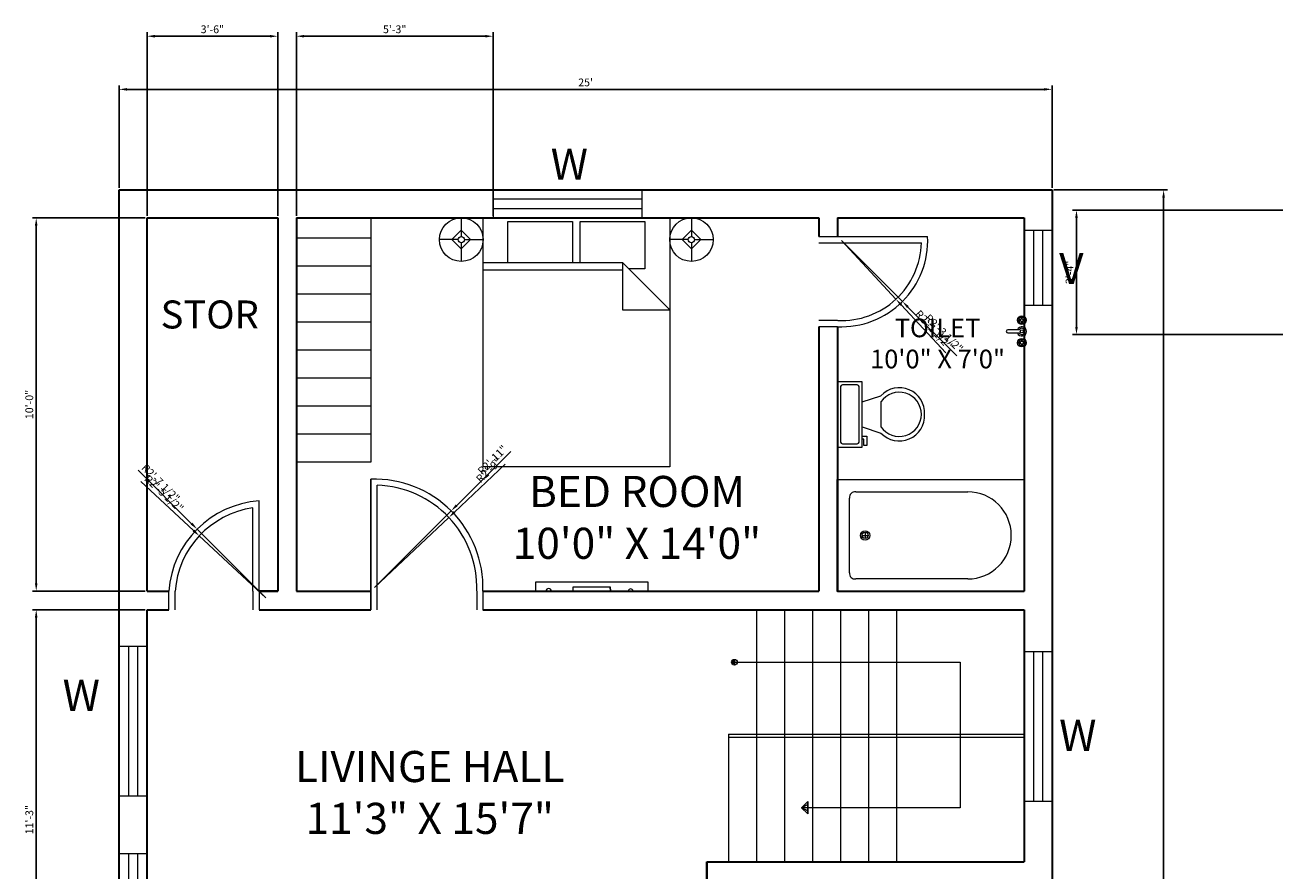
# Model space of a CAD drawing. Units: inches. Extents: x 2318 to 3542, y 1525 to 2117.
# Tile 4 of 6: x 2767 to 3169, y 1816 to 2088. Entities that reach past the tile are written whole.
import ezdxf

# ---------------------------------------------------------------- set-up
doc = ezdxf.new("R2010")
doc.units = ezdxf.units.IN
for name, color, linetype, lineweight in [('A-ANNO-DIMS', 2, 'Continuous', 18), ('A-ANNO-SYMB', 2, 'Continuous', 13), ('A-ANNO-TEXT', 7, 'Continuous', 18), ('A-AREA-IDEN', 7, 'Continuous', 25), ('A-DOOR', 4, 'Continuous', 18), ('A-EQPM', 9, 'Continuous', 18), ('A-FLOR-CASE', 8, 'Continuous', 18), ('A-FLOR-FIXT', 9, 'Continuous', 18), ('A-FLOR-STRS', 3, 'Continuous', 18), ('A-FURN', 8, 'Continuous', 18), ('A-GLAZ', 4, 'Continuous', 18), ('A-WALL', 7, 'Continuous', 35)]:
    doc.layers.add(name, color=color, linetype=linetype, lineweight=lineweight)
doc.styles.add('Annotative', font='arial.ttf')
doc.styles.get("Standard").update_dxf_attribs({"font": 'arial.ttf'})
doc.dimstyles.new('ISO-25', dxfattribs={"dimtxt": 2.5, "dimasz": 2.5, "dimexe": 1.25, "dimexo": 0.625, "dimtad": 1, "dimdec": 0, "dimlunit": 3, "dimtxsty": 'Standard', "dimcen": 2.5, "dimadec": 0, "dimazin": 0, "dimtfac": 1, "dimtdec": 0, "dimtmove": 0, "dimatfit": 3, "dimfxl": 1, "dimarcsym": 0})

# ---------------------------------------------------------------- blocks, each defined once
blk = doc.blocks.new('*D17')
at = {"layer": 'A-ANNO-DIMS', "color": 0, "lineweight": -2, "transparency": 16777216}
for p, q in [((2797.41, 2035.22), (2797.41, 2068.17)), ((2799.91, 2066.92), (3094.91, 2066.92)), ((3097.41, 2035.22), (3097.41, 2068.17))]:
    blk.add_line(p, q, dxfattribs=at)
at = {"layer": 'A-ANNO-DIMS', "color": 0, "transparency": 16777216}
for points in [[(2799.91, 2067.33), (2799.91, 2066.5), (2797.41, 2066.92)], [(3094.91, 2067.33), (3094.91, 2066.5), (3097.41, 2066.92)]]:
    blk.add_solid(points, dxfattribs=at)
at = {"layer": 'Defpoints', "color": 0, "transparency": 16777216}
for p in [(3097.41, 2066.92), (2797.41, 2034.59), (3097.41, 2034.59)]:
    blk.add_point(p, dxfattribs=at)
at = {"layer": 'A-ANNO-DIMS', "color": 0, "transparency": 16777216, "insert": (2947.41, 2068.82), "char_height": 2.5, "attachment_point": 5}
blk.add_mtext("25'", dxfattribs=at)
blk = doc.blocks.new('*D18')
at = {"layer": 'A-ANNO-DIMS', "color": 0, "lineweight": -2, "transparency": 16777216}
for p, q in [((3098.03, 2034.59), (3134.53, 2034.59)), ((3133.28, 2032.09), (3133.28, 1557.09)), ((3098.03, 1554.59), (3134.53, 1554.59))]:
    blk.add_line(p, q, dxfattribs=at)
at = {"layer": 'A-ANNO-DIMS', "color": 0, "transparency": 16777216}
for points in [[(3132.86, 2032.09), (3133.69, 2032.09), (3133.28, 2034.59)], [(3132.86, 1557.09), (3133.69, 1557.09), (3133.28, 1554.59)]]:
    blk.add_solid(points, dxfattribs=at)
at = {"layer": 'Defpoints', "color": 0, "transparency": 16777216}
for p in [(3097.41, 2034.59), (3097.41, 1554.59), (3133.28, 1554.59)]:
    blk.add_point(p, dxfattribs=at)
at = {"layer": 'A-ANNO-DIMS', "color": 0, "transparency": 16777216, "insert": (3131.38, 1794.59), "char_height": 2.5, "attachment_point": 5, "rotation": 90}
blk.add_mtext("40'", dxfattribs=at)
blk = doc.blocks.new('Bed - Queen')
for p, q in [((0, -80.00003), (0, 0)), ((0, 0), (59.99999, 0)), ((59.99999, 0), (59.99999, -80.00003)), ((7.99999, -1.2), (28.79998, -1.2)), ((7.99999, -14.4), (7.99999, -1.2)), ((28.79998, -1.2), (28.79998, -14.4)), ((31.19999, -1.2), (51.99999, -1.2)), ((31.19999, -14.4), (31.19999, -1.2)), ((51.99999, -1.2), (51.99999, -16.4)), ((0, -14.4), (44.8, -14.4)), ((59.99999, -29.6), (44.8, -14.4)), ((44.8, -14.4), (44.8, -29.6)), ((44.8, -16.8), (0, -16.8)), ((51.99999, -16.4), (46.79936, -16.4)), ((44.8, -29.6), (59.99999, -29.6)), ((59.99999, -80.00003), (0, -80.00003))]:
    blk.add_line(p, q)
blk = doc.blocks.new('Lamp - Table')
for p, q in [((0, 7), (0, 1)), ((-1, 0), (-7, 0)), ((0, 3), (-3, 0)), ((-3, 0), (0, -3)), ((3, 0), (0, 3)), ((0, -3), (3, 0)), ((1, 0), (7, 0)), ((0, -1), (0, -7))]:
    blk.add_line(p, q)
for radius in [7, 1]:
    blk.add_circle((0, 0), radius)
blk = doc.blocks.new('Bath Tub - 26 x 60 in.')
for p, q in [((8, -18), (10, -18)), ((9, -17), (9, -19))]:
    blk.add_line(p, q)
blk.add_lwpolyline([(0, -36), (0, 0), (60, 0), (60, -36)], close=True)
for points in [[(6, -4), (42, -4)], [(4, -30), (4, -6)], [(42, -32), (6, -32)]]:
    blk.add_lwpolyline(points)
for radius in [1.5, 1]:
    blk.add_circle((9, -18), radius)
for centre, radius, start, end in [((5.75, -5.75), 1.77, 81.8699, 188.1301), ((42, -18), 14, 270, 90), ((5.75, -30.25), 1.77, 171.8699, 278.1301)]:
    blk.add_arc(centre, radius, start, end)
blk = doc.blocks.new('*U14')
for p, q in [((241.3, -152.4), (241.3, -50.8)), ((-203.2, -215.9), (-203.2, -203.2)), ((-177.8, -203.2), (-177.8, -241.3)), ((-101.6, -203.2), (-152.4, -355.6)), ((101.6, -203.2), (152.4, -355.6)), ((-254, -215.9), (-203.2, -215.9)), ((-254, -241.3), (-254, -215.9)), ((-177.8, -241.3), (-254, -241.3)), ((101.6, -355.6), (-101.6, -355.6))]:
    blk.add_line(p, q)
blk.add_lwpolyline([(266.7, -203.2), (266.7, 0), (-266.7, 0), (-266.7, -203.2)], close=True)
for points in [[(-241.3, -50.8), (-241.3, -152.4)], [(215.9, -25.4), (-215.9, -25.4)], [(-215.9, -177.8), (215.9, -177.8)]]:
    blk.add_lwpolyline(points)
for centre, radius, start, end in [((-219.075, -47.625), 22.45064, 81.8699, 188.1301), ((219.075, -47.625), 22.45064, 351.8699, 98.1301), ((-219.075, -155.575), 22.45064, 171.869898, 278.1301), ((219.075, -155.575), 22.45064, 261.8699, 8.1301), ((-12.12088, -505.93752), 205.61935, 133.01722, 273.38), ((0.94996, -504.77674), 181.02486, 124.50543, 269.7), ((-0.94742, -504.77674), 181.02486, 270.3, 55.4946), ((12.12342, -505.93752), 205.61935, 266.62, 46.9828)]:
    blk.add_arc(centre, radius, start, end)
blk = doc.blocks.new('Faucet - Bathroom top')
for p, q in [((-4.107, 0.125), (-4.375, 0.125)), ((-3.75, 0.4788), (-3.75, 0.75)), ((-3.5, 0.482), (-3.5, 0.75)), ((-3.1461, 0.125), (-2.875, 0.125)), ((3.143, 0.125), (2.875, 0.125)), ((3.5, 0.4788), (3.5, 0.75)), ((3.75, 0.482), (3.75, 0.75)), ((4.1039, 0.125), (4.375, 0.125)), ((-4.1039, -0.125), (-4.375, -0.125)), ((-3.75, -0.4821), (-3.75, -0.75)), ((-3.5, -0.4789), (-3.5, -0.75)), ((-3.143, -0.125), (-2.875, -0.125)), ((-0.5, -0.8639), (-0.5, -4.5)), ((0.5, -4.5), (0.5, -0.8631)), ((3.1461, -0.125), (2.875, -0.125)), ((3.5, -0.4821), (3.5, -0.75)), ((3.75, -0.4789), (3.75, -0.75)), ((4.107, -0.125), (4.375, -0.125))]:
    blk.add_line(p, q)
for centre, radius in [((-3.625, 0), 1.375), ((-4.625, 0), 0.2795), ((-3.625, 0), 0.5), ((-3.625, 1), 0.2795), ((-2.625, 0), 0.2795), ((0, 0), 0.5), ((3.625, 0), 1.375), ((2.625, 0), 0.2795), ((3.625, 0), 0.5), ((3.625, 1), 0.2795), ((4.625, 0), 0.2795), ((-3.625, -1), 0.2795), ((3.625, -1), 0.2795)]:
    blk.add_circle(centre, radius)
for centre, radius, start, end in [((-3.625, 0), 1, 105.2407, 164.2093), ((-3.625, 0), 1, 16.44125, 74.07887), ((0, 0), 1.5, 289.6514, 250.3603), ((0, 0), 1, 300.3431, 239.7554), ((3.625, 0), 1, 106.12, 164.0884), ((3.625, 0), 1, 16.23422, 73.90469), ((-3.625, 0), 1, 196.2342, 253.9047), ((-3.625, 0), 1, 286.12, 344.0884), ((3.625, 0), 1, 196.4413, 254.0789), ((3.625, 0), 1, 285.2407, 344.2093), ((0, -4.5), 0.5, 180, 0)]:
    blk.add_arc(centre, radius, start, end)
blk = doc.blocks.new('WIN-48x9')
for p, q in [((48, 9), (0, 9)), ((0, 9), (0, 0)), ((48, 0), (48, 9)), ((48, 6), (0, 6)), ((0, 3), (48, 3)), ((0, 0), (48, 0))]:
    blk.add_line(p, q)
blk = doc.blocks.new('VENT-24x9')
for p, q in [((0, 24), (0, 0)), ((9, 24), (0, 24)), ((3, 24), (3, 0)), ((6, 0), (6, 24)), ((9, 0), (9, 24)), ((0, 0), (9, 0))]:
    blk.add_line(p, q)
blk = doc.blocks.new('TV-36-WALL')
for p, q in [((0, 0), (0, 3)), ((0, 3), (36, 3)), ((0, 0), (0, 0)), ((0, 0), (24, 0)), ((0, 0), (12, 0)), ((12, 0), (12, 1.44)), ((12, 1.44), (23.97, 1.44)), ((23.97, 1.44), (24, 0)), ((24, 0), (23.97, 1.44)), ((36, 0), (24, 0)), ((36, 3), (36, 0))]:
    blk.add_line(p, q)
for centre, radius in [((4.16, 0), 0.848), ((30.54, 0), 0.733)]:
    blk.add_arc(centre, radius, 360, 180)
blk = doc.blocks.new('*D50')
at = {"layer": 'A-ANNO-DIMS', "color": 0, "lineweight": -2, "transparency": 16777216}
for p, q in [((2806.41, 2026.22), (2806.41, 2085.25)), ((2808.91, 2084), (2845.91, 2084)), ((2848.41, 2026.22), (2848.41, 2085.25))]:
    blk.add_line(p, q, dxfattribs=at)
at = {"layer": 'A-ANNO-DIMS', "color": 0, "transparency": 16777216}
for points in [[(2808.91, 2084.42), (2808.91, 2083.58), (2806.41, 2084)], [(2845.91, 2084.42), (2845.91, 2083.58), (2848.41, 2084)]]:
    blk.add_solid(points, dxfattribs=at)
at = {"layer": 'Defpoints', "color": 0, "transparency": 16777216}
for p in [(2848.41, 2084), (2806.41, 2025.59), (2848.41, 2025.59)]:
    blk.add_point(p, dxfattribs=at)
at = {"layer": 'A-ANNO-DIMS', "color": 0, "transparency": 16777216, "insert": (2827.41, 2085.9), "char_height": 2.5, "attachment_point": 5}
blk.add_mtext('3\'-6"', dxfattribs=at)
blk = doc.blocks.new('*D56')
at = {"layer": 'A-ANNO-DIMS', "color": 0, "lineweight": -2, "transparency": 16777216}
for p, q in [((3178.81, 2028.09), (3104.01, 2028.09)), ((3105.26, 2025.59), (3105.26, 1990.55)), ((3236.71, 1988.05), (3104.01, 1988.05))]:
    blk.add_line(p, q, dxfattribs=at)
at = {"layer": 'A-ANNO-DIMS', "color": 0, "transparency": 16777216}
for points in [[(3104.85, 2025.59), (3105.68, 2025.59), (3105.26, 2028.09)], [(3104.85, 1990.55), (3105.68, 1990.55), (3105.26, 1988.05)]]:
    blk.add_solid(points, dxfattribs=at)
at = {"layer": 'Defpoints', "color": 0, "transparency": 16777216}
for p in [(3179.43, 2028.09), (3105.26, 1988.05), (3237.33, 1988.05)]:
    blk.add_point(p, dxfattribs=at)
at = {"layer": 'A-ANNO-DIMS', "color": 0, "transparency": 16777216, "insert": (3103.36, 2008.07), "char_height": 2.5, "attachment_point": 5, "rotation": 90}
blk.add_mtext('3\'-4"', dxfattribs=at)
blk = doc.blocks.new('*D62')
at = {"layer": 'A-ANNO-DIMS', "color": 0, "lineweight": -2, "transparency": 16777216}
for p, q in [((2805.78, 2025.59), (2769.51, 2025.59)), ((2770.76, 1908.09), (2770.76, 2023.09)), ((2805.78, 1905.59), (2769.51, 1905.59))]:
    blk.add_line(p, q, dxfattribs=at)
at = {"layer": 'A-ANNO-DIMS', "color": 0, "transparency": 16777216}
for points in [[(2770.34, 2023.09), (2771.17, 2023.09), (2770.76, 2025.59)], [(2770.34, 1908.09), (2771.17, 1908.09), (2770.76, 1905.59)]]:
    blk.add_solid(points, dxfattribs=at)
at = {"layer": 'Defpoints', "color": 0, "transparency": 16777216}
for p in [(2770.76, 2025.59), (2806.41, 2025.59), (2806.41, 1905.59)]:
    blk.add_point(p, dxfattribs=at)
at = {"layer": 'A-ANNO-DIMS', "color": 0, "transparency": 16777216, "insert": (2768.86, 1965.59), "char_height": 2.5, "attachment_point": 5, "rotation": 90}
blk.add_mtext('10\'-0"', dxfattribs=at)
blk = doc.blocks.new('*D63')
at = {"layer": 'A-ANNO-DIMS', "color": 0, "lineweight": -2, "transparency": 16777216}
for p, q in [((2805.78, 1899.59), (2769.51, 1899.59)), ((2770.76, 1767.09), (2770.76, 1897.09)), ((2805.78, 1764.59), (2769.51, 1764.59))]:
    blk.add_line(p, q, dxfattribs=at)
at = {"layer": 'A-ANNO-DIMS', "color": 0, "transparency": 16777216}
for points in [[(2770.34, 1897.09), (2771.17, 1897.09), (2770.76, 1899.59)], [(2770.34, 1767.09), (2771.17, 1767.09), (2770.76, 1764.59)]]:
    blk.add_solid(points, dxfattribs=at)
at = {"layer": 'Defpoints', "color": 0, "transparency": 16777216}
for p in [(2770.76, 1899.59), (2806.41, 1899.59), (2806.41, 1764.59)]:
    blk.add_point(p, dxfattribs=at)
at = {"layer": 'A-ANNO-DIMS', "color": 0, "transparency": 16777216, "insert": (2768.86, 1832.09), "char_height": 2.5, "attachment_point": 5, "rotation": 90}
blk.add_mtext('11\'-3"', dxfattribs=at)
blk = doc.blocks.new('*D72')
at = {"layer": 'A-ANNO-DIMS', "color": 0, "lineweight": -2, "transparency": 16777216}
for p, q in [((2854.41, 2026.22), (2854.41, 2085.25)), ((2856.91, 2084), (2915.15, 2084)), ((2917.65, 2026.22), (2917.65, 2085.25))]:
    blk.add_line(p, q, dxfattribs=at)
at = {"layer": 'A-ANNO-DIMS', "color": 0, "transparency": 16777216}
for points in [[(2856.91, 2084.42), (2856.91, 2083.58), (2854.41, 2084)], [(2915.15, 2084.42), (2915.15, 2083.58), (2917.65, 2084)]]:
    blk.add_solid(points, dxfattribs=at)
at = {"layer": 'Defpoints', "color": 0, "transparency": 16777216}
for p in [(2917.65, 2084), (2854.41, 2025.59), (2917.65, 2025.59)]:
    blk.add_point(p, dxfattribs=at)
at = {"layer": 'A-ANNO-DIMS', "color": 0, "transparency": 16777216, "insert": (2886.03, 2085.9), "char_height": 2.5, "attachment_point": 5}
blk.add_mtext('5\'-3"', dxfattribs=at)
blk = doc.blocks.new('*D82')
at = {"layer": 'A-ANNO-DIMS', "color": 0, "lineweight": -2, "transparency": 16777216}
for p, q in [((2923.33, 1950.52), (2905.97, 1933.15)), ((2879.52, 1906.7), (2904.2, 1931.39))]:
    blk.add_line(p, q, dxfattribs=at)
at = {"layer": 'A-ANNO-DIMS', "color": 0, "transparency": 16777216}
blk.add_solid([(2905.67, 1933.45), (2906.26, 1932.86), (2904.2, 1931.39)], dxfattribs=at)
at = {"layer": 'Defpoints', "color": 0, "transparency": 16777216}
for p in [(2904.2, 1931.39), (2879.52, 1906.7)]:
    blk.add_point(p, dxfattribs=at)
at = {"layer": 'A-ANNO-DIMS', "color": 0, "transparency": 16777216, "insert": (2917.68, 1947.53), "char_height": 2.5, "attachment_point": 5, "rotation": 45}
blk.add_mtext('R2\'-11"', dxfattribs=at)
blk = doc.blocks.new('*D83')
at = {"layer": 'A-ANNO-DIMS', "color": 0, "lineweight": -2, "transparency": 16777216}
for p, q in [((2803.52, 1944.48), (2820.73, 1927.27)), ((2844.63, 1903.37), (2822.5, 1925.5))]:
    blk.add_line(p, q, dxfattribs=at)
at = {"layer": 'A-ANNO-DIMS', "color": 0, "transparency": 16777216}
blk.add_solid([(2821.02, 1927.57), (2820.43, 1926.98), (2822.5, 1925.5)], dxfattribs=at)
at = {"layer": 'Defpoints', "color": 0, "transparency": 16777216}
for p in [(2822.5, 1925.5), (2844.63, 1903.37)]:
    blk.add_point(p, dxfattribs=at)
at = {"layer": 'A-ANNO-DIMS', "color": 0, "transparency": 16777216, "insert": (2810.57, 1940.14), "char_height": 2.5, "attachment_point": 5, "rotation": 314.9995}
blk.add_mtext('R2\'-7 1/2"', dxfattribs=at)
blk = doc.blocks.new('*D85')
at = {"layer": 'A-ANNO-DIMS', "color": 0, "lineweight": -2, "transparency": 16777216}
for p, q in [((3029.69, 2018.31), (3049.31, 1998.69)), ((3066.78, 1981.22), (3051.08, 1996.92))]:
    blk.add_line(p, q, dxfattribs=at)
at = {"layer": 'A-ANNO-DIMS', "color": 0, "transparency": 16777216}
blk.add_solid([(3051.37, 1997.22), (3050.78, 1996.63), (3049.31, 1998.69)], dxfattribs=at)
at = {"layer": 'Defpoints', "color": 0, "transparency": 16777216}
for p in [(3029.69, 2018.31), (3049.31, 1998.69)]:
    blk.add_point(p, dxfattribs=at)
at = {"layer": 'A-ANNO-DIMS', "color": 0, "transparency": 16777216, "insert": (3062.44, 1988.27), "char_height": 2.5, "attachment_point": 5, "rotation": 315.0005}
blk.add_mtext('R2\'-3 1/2"', dxfattribs=at)
blk = doc.blocks.new('*D100')
at = {"layer": 'A-ANNO-DIMS', "color": 0, "lineweight": -2, "transparency": 16777216}
for p, q in [((2804.42, 1940.81), (2821.36, 1925.04)), ((2844.63, 1903.37), (2823.19, 1923.34))]:
    blk.add_line(p, q, dxfattribs=at)
at = {"layer": 'A-ANNO-DIMS', "color": 0, "transparency": 16777216}
blk.add_solid([(2821.64, 1925.35), (2821.07, 1924.74), (2823.19, 1923.34)], dxfattribs=at)
at = {"layer": 'Defpoints', "color": 0, "transparency": 16777216}
for p in [(2823.19, 1923.34), (2844.63, 1903.37)]:
    blk.add_point(p, dxfattribs=at)
at = {"layer": 'A-ANNO-DIMS', "color": 0, "transparency": 16777216, "insert": (2811.63, 1936.72), "char_height": 2.5, "attachment_point": 5, "rotation": 317.0392}
blk.add_mtext('R2\'-5 1/2"', dxfattribs=at)
blk = doc.blocks.new('*D109')
at = {"layer": 'A-ANNO-DIMS', "color": 0, "lineweight": -2, "transparency": 16777216}
for p, q in [((2921.57, 1946.35), (2905.28, 1930.99)), ((2879.52, 1906.7), (2903.46, 1929.28))]:
    blk.add_line(p, q, dxfattribs=at)
at = {"layer": 'A-ANNO-DIMS', "color": 0, "transparency": 16777216}
blk.add_solid([(2904.99, 1931.3), (2905.57, 1930.69), (2903.46, 1929.28)], dxfattribs=at)
at = {"layer": 'Defpoints', "color": 0, "transparency": 16777216}
for p in [(2903.46, 1929.28), (2879.52, 1906.7)]:
    blk.add_point(p, dxfattribs=at)
at = {"layer": 'A-ANNO-DIMS', "color": 0, "transparency": 16777216, "insert": (2916.52, 1944.21), "char_height": 2.5, "attachment_point": 5, "rotation": 43.3143}
blk.add_mtext('R2\'-9"', dxfattribs=at)
blk = doc.blocks.new('*D111')
at = {"layer": 'A-ANNO-DIMS', "color": 0, "lineweight": -2, "transparency": 16777216}
for p, q in [((3029.69, 2018.31), (3047.21, 1999.44)), ((3063.2, 1982.22), (3048.91, 1997.61))]:
    blk.add_line(p, q, dxfattribs=at)
at = {"layer": 'A-ANNO-DIMS', "color": 0, "transparency": 16777216}
blk.add_solid([(3049.22, 1997.89), (3048.61, 1997.32), (3047.21, 1999.44)], dxfattribs=at)
at = {"layer": 'Defpoints', "color": 0, "transparency": 16777216}
for p in [(3029.69, 2018.31), (3047.21, 1999.44)]:
    blk.add_point(p, dxfattribs=at)
at = {"layer": 'A-ANNO-DIMS', "color": 0, "transparency": 16777216, "insert": (3059.12, 1989.43), "char_height": 2.5, "attachment_point": 5, "rotation": 312.8754}
blk.add_mtext('R2\'-1 1/2"', dxfattribs=at)

msp = doc.modelspace()

# ---------------------------------------------------------------- linework, layer by layer
at = {"layer": 'A-ANNO-SYMB'}
for p, q in [((2995.27, 1882.73), (2994.36, 1882.73)), ((2994.36, 1882.73), (2995.27, 1882.73)), ((2995.27, 1882.73), (2994.61, 1882.11)), ((2995.27, 1882.73), (2994.73, 1883.45)), ((2994.73, 1883.45), (2995.27, 1882.73)), ((2995.27, 1882.73), (2995.27, 1883.64)), ((2995.27, 1883.64), (2995.27, 1881.82)), ((2995.27, 1882.73), (3067.85, 1882.73)), ((2995.27, 1881.82), (2995.27, 1882.73)), ((3067.85, 1882.73), (3067.85, 1835.92)), ((3016.89, 1835.92), (3018.89, 1837.92)), ((3016.89, 1835.92), (3018.89, 1836.92)), ((3018.89, 1836.92), (3016.89, 1835.92)), ((3018.89, 1835.92), (3018.89, 1837.92)), ((3018.89, 1837.92), (3018.89, 1835.92)), ((3018.89, 1837.92), (3018.89, 1833.92)), ((3018.89, 1835.92), (3016.89, 1835.92)), ((3018.89, 1833.92), (3016.89, 1835.92)), ((3016.89, 1835.92), (3018.89, 1834.92)), ((3018.89, 1834.92), (3016.89, 1835.92)), ((3020.41, 1835.92), (3018.89, 1835.92)), ((3018.89, 1835.92), (3018.89, 1833.92)), ((3018.89, 1833.92), (3018.89, 1835.92)), ((3067.85, 1835.92), (3020.41, 1835.92))]:
    msp.add_line(p, q, dxfattribs=at)
msp.add_circle((2995.27, 1882.73), 0.906, dxfattribs=at)
at = {"layer": 'A-DOOR'}
for p, q in [((3022.41, 2019.59), (3028.41, 2019.59)), ((3022.41, 2019.59), (3028.41, 2019.59)), ((3028.41, 2019.59), (3057.41, 2019.59)), ((3022.41, 2017.59), (3028.41, 2017.59)), ((3028.41, 2017.59), (3055.43, 2017.59)), ((3028.41, 1992.59), (3022.41, 1992.59)), ((3028.41, 1990.59), (3022.41, 1990.59)), ((2878.41, 1929.59), (2878.41, 1941.59)), ((2878.41, 1941.59), (2878.41, 1905.59)), ((2880.41, 1929.59), (2880.41, 1939.6)), ((2842.41, 1905.59), (2842.41, 1934.59)), ((2840.41, 1905.59), (2840.41, 1932.37)), ((2878.41, 1905.59), (2878.41, 1929.59)), ((2878.41, 1929.59), (2878.41, 1905.59)), ((2878.41, 1905.59), (2878.41, 1929.59)), ((2880.41, 1905.59), (2880.41, 1929.59)), ((2813.41, 1899.59), (2813.41, 1905.59)), ((2815.41, 1899.59), (2815.41, 1905.59)), ((2840.41, 1905.59), (2840.41, 1899.59)), ((2842.41, 1905.59), (2842.41, 1899.59)), ((2878.41, 1905.59), (2878.41, 1899.59)), ((2878.41, 1899.59), (2878.41, 1905.59)), ((2878.41, 1899.59), (2878.41, 1905.59)), ((2880.41, 1899.59), (2880.41, 1905.59)), ((2912.41, 1905.59), (2912.41, 1899.59)), ((2914.41, 1905.59), (2914.41, 1899.59))]:
    msp.add_line(p, q, dxfattribs=at)
for centre, radius, start, end in [((3029.69, 2018.31), 27.74, 267.3408, 2.6592), ((3029.69, 2018.31), 25.74, 267.3408, 358.4131), ((2879.52, 1906.7), 34.91, 358.177, 91.823), ((2879.52, 1906.7), 32.91, 358.177, 88.4511), ((2844.63, 1903.37), 31.3, 94.0761, 175.9239), ((2844.63, 1903.37), 29.3, 98.29, 175.787)]:
    msp.add_arc(centre, radius, start, end, dxfattribs=at)
at = {"layer": 'A-FLOR-CASE'}
for p, q in [((2878.41, 2025.59), (2878.41, 1947.03)), ((2878.41, 2019.03), (2854.41, 2019.03)), ((2878.41, 2010.03), (2854.41, 2010.03)), ((2878.41, 2001.03), (2854.41, 2001.03)), ((2878.41, 1992.03), (2854.41, 1992.03)), ((2878.41, 1983.03), (2854.41, 1983.03)), ((2878.41, 1974.03), (2854.41, 1974.03)), ((2878.41, 1965.03), (2854.41, 1965.03)), ((2878.41, 1956.03), (2854.41, 1956.03)), ((2878.41, 1947.03), (2854.41, 1947.03))]:
    msp.add_line(p, q, dxfattribs=at)
at = {"layer": 'A-FLOR-STRS'}
for p, q in [((3002.41, 1899.59), (3002.41, 1818.59)), ((3011.41, 1899.59), (3011.41, 1818.59)), ((3020.41, 1899.59), (3020.41, 1818.59)), ((3029.41, 1899.59), (3029.41, 1818.59)), ((3038.41, 1899.59), (3038.41, 1818.59)), ((3047.41, 1899.59), (3047.41, 1818.59)), ((2993.41, 1859.59), (3088.41, 1859.59)), ((2993.41, 1859.59), (2993.41, 1818.59)), ((2993.41, 1858.59), (3088.41, 1858.59))]:
    msp.add_line(p, q, dxfattribs=at)
at = {"layer": 'A-WALL'}
for p, q in [((2797.41, 2034.59), (3097.41, 2034.59)), ((2797.41, 1554.59), (2797.41, 2034.59)), ((3097.41, 2034.59), (3097.41, 1554.59)), ((2806.41, 2025.59), (2848.41, 2025.59)), ((2806.41, 1905.59), (2806.41, 2025.59)), ((2848.41, 2025.59), (2848.41, 1905.59)), ((2854.41, 2025.59), (2854.41, 1905.59)), ((2854.41, 2025.59), (3022.41, 2025.59)), ((3022.41, 2025.59), (3022.41, 2019.59)), ((3022.41, 2025.59), (3022.41, 2019.59)), ((3028.41, 2025.59), (3028.41, 2019.59)), ((3028.41, 2025.59), (3088.41, 2025.59)), ((3088.41, 2025.59), (3088.41, 1905.59)), ((3022.41, 1990.59), (3022.41, 1905.59)), ((3028.41, 1990.59), (3028.41, 1905.59)), ((2806.41, 1905.59), (2813.41, 1905.59)), ((2848.41, 1905.59), (2842.41, 1905.59)), ((2842.41, 1905.59), (2848.41, 1905.59)), ((2854.41, 1905.59), (2878.41, 1905.59)), ((2854.41, 1905.59), (2878.41, 1905.59)), ((2914.41, 1905.59), (3022.41, 1905.59)), ((3028.41, 1905.59), (3088.41, 1905.59)), ((2806.41, 1899.59), (2813.41, 1899.59)), ((2806.41, 1764.59), (2806.41, 1899.59)), ((2842.41, 1899.59), (2878.41, 1899.59)), ((2914.41, 1899.59), (3088.41, 1899.59)), ((3088.41, 1899.59), (3088.41, 1818.59)), ((2986.41, 1818.59), (3088.41, 1818.59)), ((2986.41, 1812.59), (2986.41, 1818.59)), ((2986.41, 1818.59), (2986.41, 1764.59))]:
    msp.add_line(p, q, dxfattribs=at)

# ---------------------------------------------------------------- block references
at = {"layer": 'A-EQPM'}
msp.add_blockref('TV-36-WALL', (2931.38, 1905.57), dxfattribs=at)
at = {"layer": 'A-FLOR-FIXT', "rotation": 270}
msp.add_blockref('Faucet - Bathroom top', (3087.7, 1989.09), dxfattribs=at)
at = {"layer": 'A-FLOR-FIXT', "xscale": 0.0393700787401575, "yscale": 0.0393700787401575, "zscale": 0.0393700787401575, "rotation": 90}
msp.add_blockref('*U14', (3028.39, 1962.42), dxfattribs=at)
at = {"layer": 'A-FLOR-FIXT'}
msp.add_blockref('Bath Tub - 26 x 60 in.', (3028.3, 1941.5), dxfattribs=at)
at = {"layer": 'A-FURN'}
for name, p in [('Lamp - Table', (2907.45, 2018.59)), ('Bed - Queen', (2914.45, 2025.59)), ('Lamp - Table', (2981.45, 2018.59))]:
    msp.add_blockref(name, p, dxfattribs=at)
at = {"layer": 'A-GLAZ'}
msp.add_blockref('WIN-48x9', (2917.65, 2025.59), dxfattribs=at)
for name, p, rotation in [('VENT-24x9', (3097.41, 2021.53), 180), ('WIN-48x9', (2806.41, 1839.78), 90.0000000000021), ('WIN-48x9', (3097.41, 1838.08), 89.99999999999969), ('WIN-48x9', (2806.41, 1773.07), 90.00000000000179)]:
    msp.add_blockref(name, p, dxfattribs=dict(at, rotation=rotation))

# ---------------------------------------------------------------- texts
at = {"layer": 'A-ANNO-TEXT', "char_height": 10, "attachment_point": 1}
for s, insert in [('\\pxt1;W', (2936.2, 2047.85)), ('\\pxt1;V', (3099.69, 2014.29)), ('\\pxt1;W', (2779.26, 1877.08)), ('\\pxt1;W', (3099.7, 1864.2))]:
    msp.add_mtext_dynamic_manual_height_columns(s, width=219.3474, gutter_width=12.5, heights=[0], dxfattribs=dict(at, insert=insert))
at = {"layer": 'A-AREA-IDEN', "attachment_point": 1}
for s, width, insert, char_height in [('STOR', 31.8275, (2810.76, 1999.03), 9), ('\\pxqc,t2;TOILET\\P10\'0" X 7\'0"', 46.835, (3037.17, 1993.21), 6)]:
    msp.add_mtext_dynamic_manual_height_columns(s, width=width, gutter_width=12.5, heights=[0], dxfattribs=dict(at, insert=insert, char_height=char_height))
at = {"layer": 'A-AREA-IDEN', "char_height": 10, "width": 132.7792, "attachment_point": 1, "style": 'Annotative'}
for s, insert in [('\\pxqc;BED ROOM\\P10\'0" X 14\'0"', (2897.54, 1942.63)), ('\\pxqc;LIVINGE HALL\\P11\'3" X 15\'7"', (2830.91, 1854.18))]:
    msp.add_mtext(s, dxfattribs=dict(at, insert=insert))

# ---------------------------------------------------------------- dimensions: what is measured, and where the dimension line sits
at = {"layer": 'A-ANNO-DIMS'}
for base, p1, p2, override, picture, middle in [((2848.41, 2084), (2806.41, 2025.59), (2848.41, 2025.59), {"dimdec": 1, "dimlfac": 1, "dimrnd": 0, "dimzin": 1, "dimdsep": 46, "dimlunit": 4, "dimfrac": 2}, '*D50', (2827.41, 2085.9)), ((2917.65, 2084), (2854.41, 2025.59), (2917.65, 2025.59), {"dimdec": 1, "dimlfac": 1, "dimrnd": 0, "dimzin": 1, "dimdsep": 46, "dimlunit": 4, "dimfrac": 2}, '*D72', (2886.03, 2085.9)), ((3097.41, 2066.92), (2797.41, 2034.59), (3097.41, 2034.59), {"dimclrd": 0, "dimclre": 0, "dimclrt": 0}, '*D17', (2947.41, 2068.82))]:
    dim = msp.add_linear_dim(base=base, p1=p1, p2=p2, dimstyle='ISO-25', override=override, dxfattribs=at)
    dim.commit()
    dim.dimension.update_dxf_attribs({"geometry": picture, "text_midpoint": middle})
for base, p1, p2, override, picture, middle in [((3133.28, 1554.59), (3097.41, 2034.59), (3097.41, 1554.59), {"dimclrd": 0, "dimclre": 0, "dimclrt": 0}, '*D18', (3131.38, 1794.59)), ((3105.26, 1988.05), (3179.43, 2028.09), (3237.33, 1988.05), {"dimdec": 1, "dimlfac": 1, "dimrnd": 0, "dimzin": 1, "dimdsep": 46, "dimlunit": 4, "dimfrac": 2}, '*D56', (3103.36, 2008.07)), ((2770.76, 2025.59), (2806.41, 1905.59), (2806.41, 2025.59), {"dimdec": 1, "dimlfac": 1, "dimrnd": 0, "dimzin": 1, "dimdsep": 46, "dimlunit": 4, "dimfrac": 2}, '*D62', (2768.86, 1965.59)), ((2770.76, 1899.59), (2806.41, 1764.59), (2806.41, 1899.59), {"dimdec": 1, "dimlfac": 1, "dimrnd": 0, "dimzin": 1, "dimdsep": 46, "dimlunit": 4, "dimfrac": 2}, '*D63', (2768.86, 1832.09))]:
    dim = msp.add_linear_dim(base=base, p1=p1, p2=p2, angle=90, dimstyle='ISO-25', override=override, dxfattribs=at)
    dim.commit()
    dim.dimension.update_dxf_attribs({"geometry": picture, "text_midpoint": middle})
for center, mpoint, picture, middle in [((3029.69, 2018.31), (3049.31, 1998.69), '*D85', (3061.08, 1986.92)), ((3029.69, 2018.31), (3047.21, 1999.44), '*D111', (3057.72, 1988.12)), ((2879.52, 1906.7), (2904.2, 1931.39), '*D82', (2919.01, 1946.2)), ((2844.63, 1903.37), (2822.5, 1925.5), '*D83', (2809.22, 1938.78)), ((2879.52, 1906.7), (2903.46, 1929.28), '*D109', (2917.83, 1942.82)), ((2844.63, 1903.37), (2823.19, 1923.34), '*D100', (2810.32, 1935.32))]:
    dim = msp.add_radius_dim(center=center, mpoint=mpoint, dimstyle='ISO-25', override={"dimdec": 1, "dimlfac": 1, "dimrnd": 0, "dimzin": 1, "dimdsep": 46, "dimlunit": 4, "dimfrac": 2}, dxfattribs=at)
    dim.commit()
    dim.dimension.update_dxf_attribs({"geometry": picture, "text_midpoint": middle, "dimtype": 164})

doc.saveas('drawing.dxf')
